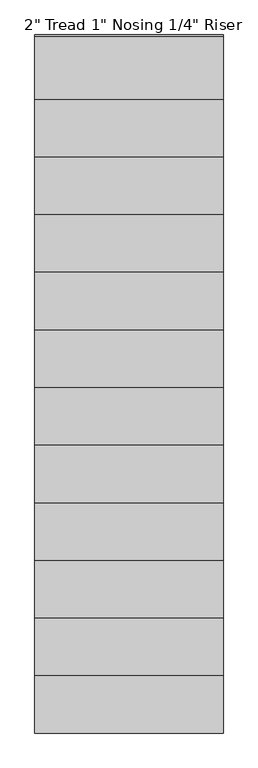
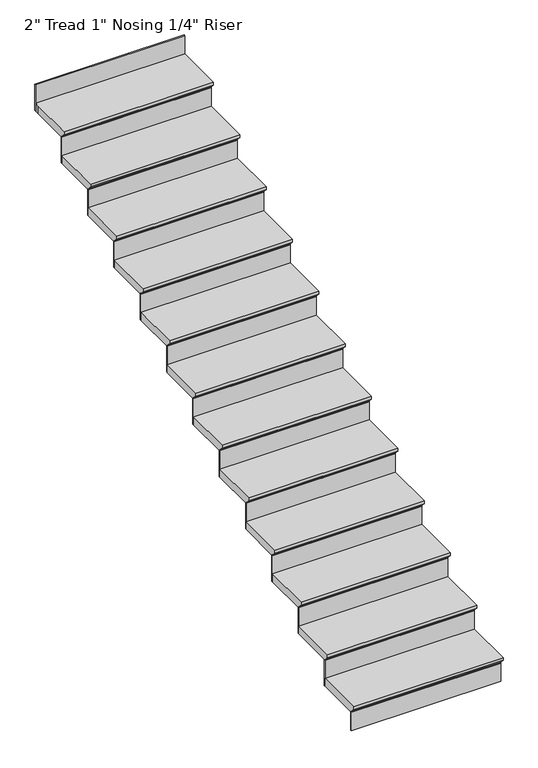
"""IFC4 building model written with IfcOpenShell, lengths in millimetres: stair flight geometry."""

from ifc_helpers import new_model, si_unit, origin, place, context, project, spatial, faceted_brep, source, transform, mapped, element, save


def stair_flight_c0f4d4ee(model_context):
    return source(origin(), model_context, "Body", "Brep", [
        faceted_brep([(-2703.0415084, 19841.9216096, 25384.9005799), (-2703.0415084, 19841.9216096, 25403.9505799), (-3617.4415084, 19841.9216096, 25403.9505799), (-3617.4415084, 19841.9216096, 25384.9005799), (-2703.0415084, 19867.3216096, 25359.5005799), (-3617.4415084, 19867.3216096, 25359.5005799), (-2703.0415084, 20146.7216096, 25403.9505799), (-3617.4415084, 20146.7216096, 25403.9505799), (-3617.4415084, 19867.3216096, 25353.1505799), (-3617.4415084, 20146.7216096, 25353.1505799), (-2703.0415084, 20146.7216096, 25353.1505799), (-2703.0415084, 19867.3216096, 25353.1505799)], [[[0, 1, 2, 3]], [[4, 0, 3, 5]], [[2, 1, 6, 7]], [[8, 9, 10, 11]], [[2, 7, 9, 8, 5, 3]], [[8, 11, 4, 5]], [[6, 1, 0, 4, 11, 10]], [[7, 6, 10, 9]]]),
        faceted_brep([(-2703.0415084, 19867.3216096, 25353.1505799), (-2703.0415084, 19867.3216096, 25234.6172466), (-2703.0415084, 19873.6716096, 25234.6172466), (-2703.0415084, 19873.6716096, 25353.1505799), (-3617.4415084, 19867.3216096, 25353.1505799), (-3617.4415084, 19873.6716096, 25353.1505799), (-3617.4415084, 19873.6716096, 25234.6172466), (-3617.4415084, 19867.3216096, 25234.6172466)], [[[0, 1, 2, 3]], [[4, 5, 6, 7]], [[1, 0, 4, 7]], [[2, 1, 7, 6]], [[3, 2, 6, 5]], [[0, 3, 5, 4]]]),
        faceted_brep([(-2703.0415084, 20146.7216096, 25522.4839133), (-2703.0415084, 20146.7216096, 25353.1505799), (-2703.0415084, 20153.0716096, 25353.1505799), (-2703.0415084, 20153.0716096, 25522.4839133), (-3617.4415084, 20146.7216096, 25522.4839133), (-3617.4415084, 20153.0716096, 25522.4839133), (-3617.4415084, 20153.0716096, 25353.1505799), (-3617.4415084, 20146.7216096, 25353.1505799)], [[[0, 1, 2, 3]], [[4, 5, 6, 7]], [[1, 0, 4, 7]], [[2, 1, 7, 6]], [[3, 2, 6, 5]], [[0, 3, 5, 4]]]),
        faceted_brep([(-3617.4415084, 20121.3216096, 25573.2839133), (-2703.0415084, 20121.3216096, 25573.2839133), (-2703.0415084, 20426.1216096, 25573.2839133), (-3617.4415084, 20426.1216096, 25573.2839133), (-3617.4415084, 20146.7216096, 25522.4839133), (-3617.4415084, 20426.1216096, 25522.4839133), (-2703.0415084, 20426.1216096, 25522.4839133), (-2703.0415084, 20146.7216096, 25522.4839133), (-3617.4415084, 20146.7216096, 25528.8339133), (-3617.4415084, 20121.3216096, 25554.2339133), (-2703.0415084, 20146.7216096, 25528.8339133), (-2703.0415084, 20121.3216096, 25554.2339133)], [[[0, 1, 2, 3]], [[4, 5, 6, 7]], [[0, 3, 5, 4, 8, 9]], [[4, 7, 10, 8]], [[2, 1, 11, 10, 7, 6]], [[3, 2, 6, 5]], [[11, 1, 0, 9]], [[10, 11, 9, 8]]]),
        faceted_brep([(-2703.0415084, 20426.1216096, 25691.8172466), (-2703.0415084, 20426.1216096, 25522.4839133), (-2703.0415084, 20432.4716096, 25522.4839133), (-2703.0415084, 20432.4716096, 25691.8172466), (-3617.4415084, 20426.1216096, 25691.8172466), (-3617.4415084, 20432.4716096, 25691.8172466), (-3617.4415084, 20432.4716096, 25522.4839133), (-3617.4415084, 20426.1216096, 25522.4839133)], [[[0, 1, 2, 3]], [[4, 5, 6, 7]], [[1, 0, 4, 7]], [[2, 1, 7, 6]], [[3, 2, 6, 5]], [[0, 3, 5, 4]]]),
        faceted_brep([(-3617.4415084, 20400.7216096, 25742.6172466), (-2703.0415084, 20400.7216096, 25742.6172466), (-2703.0415084, 20705.5216096, 25742.6172466), (-3617.4415084, 20705.5216096, 25742.6172466), (-3617.4415084, 20426.1216096, 25691.8172466), (-3617.4415084, 20705.5216096, 25691.8172466), (-2703.0415084, 20705.5216096, 25691.8172466), (-2703.0415084, 20426.1216096, 25691.8172466), (-3617.4415084, 20426.1216096, 25698.1672466), (-3617.4415084, 20400.7216096, 25723.5672466), (-2703.0415084, 20426.1216096, 25698.1672466), (-2703.0415084, 20400.7216096, 25723.5672466)], [[[0, 1, 2, 3]], [[4, 5, 6, 7]], [[0, 3, 5, 4, 8, 9]], [[4, 7, 10, 8]], [[2, 1, 11, 10, 7, 6]], [[3, 2, 6, 5]], [[11, 1, 0, 9]], [[10, 11, 9, 8]]]),
        faceted_brep([(-2703.0415084, 20705.5216096, 25861.1505799), (-2703.0415084, 20705.5216096, 25691.8172466), (-2703.0415084, 20711.8716096, 25691.8172466), (-2703.0415084, 20711.8716096, 25861.1505799), (-3617.4415084, 20705.5216096, 25861.1505799), (-3617.4415084, 20711.8716096, 25861.1505799), (-3617.4415084, 20711.8716096, 25691.8172466), (-3617.4415084, 20705.5216096, 25691.8172466)], [[[0, 1, 2, 3]], [[4, 5, 6, 7]], [[1, 0, 4, 7]], [[2, 1, 7, 6]], [[3, 2, 6, 5]], [[0, 3, 5, 4]]]),
        faceted_brep([(-3617.4415084, 20680.1216096, 25911.9505799), (-2703.0415084, 20680.1216096, 25911.9505799), (-2703.0415084, 20984.9216096, 25911.9505799), (-3617.4415084, 20984.9216096, 25911.9505799), (-3617.4415084, 20705.5216096, 25861.1505799), (-3617.4415084, 20984.9216096, 25861.1505799), (-2703.0415084, 20984.9216096, 25861.1505799), (-2703.0415084, 20705.5216096, 25861.1505799), (-3617.4415084, 20705.5216096, 25867.5005799), (-3617.4415084, 20680.1216096, 25892.9005799), (-2703.0415084, 20705.5216096, 25867.5005799), (-2703.0415084, 20680.1216096, 25892.9005799)], [[[0, 1, 2, 3]], [[4, 5, 6, 7]], [[0, 3, 5, 4, 8, 9]], [[4, 7, 10, 8]], [[2, 1, 11, 10, 7, 6]], [[3, 2, 6, 5]], [[11, 1, 0, 9]], [[10, 11, 9, 8]]]),
        faceted_brep([(-2703.0415084, 20984.9216096, 26030.4839133), (-2703.0415084, 20984.9216096, 25861.1505799), (-2703.0415084, 20991.2716096, 25861.1505799), (-2703.0415084, 20991.2716096, 26030.4839133), (-3617.4415084, 20984.9216096, 26030.4839133), (-3617.4415084, 20991.2716096, 26030.4839133), (-3617.4415084, 20991.2716096, 25861.1505799), (-3617.4415084, 20984.9216096, 25861.1505799)], [[[0, 1, 2, 3]], [[4, 5, 6, 7]], [[1, 0, 4, 7]], [[2, 1, 7, 6]], [[3, 2, 6, 5]], [[0, 3, 5, 4]]]),
        faceted_brep([(-3617.4415084, 20959.5216096, 26081.2839133), (-2703.0415084, 20959.5216096, 26081.2839133), (-2703.0415084, 21264.3216096, 26081.2839133), (-3617.4415084, 21264.3216096, 26081.2839133), (-3617.4415084, 20984.9216096, 26030.4839133), (-3617.4415084, 21264.3216096, 26030.4839133), (-2703.0415084, 21264.3216096, 26030.4839133), (-2703.0415084, 20984.9216096, 26030.4839133), (-3617.4415084, 20984.9216096, 26036.8339133), (-3617.4415084, 20959.5216096, 26062.2339133), (-2703.0415084, 20984.9216096, 26036.8339133), (-2703.0415084, 20959.5216096, 26062.2339133)], [[[0, 1, 2, 3]], [[4, 5, 6, 7]], [[0, 3, 5, 4, 8, 9]], [[4, 7, 10, 8]], [[2, 1, 11, 10, 7, 6]], [[3, 2, 6, 5]], [[11, 1, 0, 9]], [[10, 11, 9, 8]]]),
        faceted_brep([(-2703.0415084, 21264.3216096, 26199.8172466), (-2703.0415084, 21264.3216096, 26030.4839133), (-2703.0415084, 21270.6716096, 26030.4839133), (-2703.0415084, 21270.6716096, 26199.8172466), (-3617.4415084, 21264.3216096, 26199.8172466), (-3617.4415084, 21270.6716096, 26199.8172466), (-3617.4415084, 21270.6716096, 26030.4839133), (-3617.4415084, 21264.3216096, 26030.4839133)], [[[0, 1, 2, 3]], [[4, 5, 6, 7]], [[1, 0, 4, 7]], [[2, 1, 7, 6]], [[3, 2, 6, 5]], [[0, 3, 5, 4]]]),
        faceted_brep([(-3617.4415084, 21238.9216096, 26250.6172466), (-2703.0415084, 21238.9216096, 26250.6172466), (-2703.0415084, 21543.7216096, 26250.6172466), (-3617.4415084, 21543.7216096, 26250.6172466), (-3617.4415084, 21264.3216096, 26199.8172466), (-3617.4415084, 21543.7216096, 26199.8172466), (-2703.0415084, 21543.7216096, 26199.8172466), (-2703.0415084, 21264.3216096, 26199.8172466), (-3617.4415084, 21264.3216096, 26206.1672466), (-3617.4415084, 21238.9216096, 26231.5672466), (-2703.0415084, 21264.3216096, 26206.1672466), (-2703.0415084, 21238.9216096, 26231.5672466)], [[[0, 1, 2, 3]], [[4, 5, 6, 7]], [[0, 3, 5, 4, 8, 9]], [[4, 7, 10, 8]], [[2, 1, 11, 10, 7, 6]], [[3, 2, 6, 5]], [[11, 1, 0, 9]], [[10, 11, 9, 8]]]),
        faceted_brep([(-2703.0415084, 21543.7216096, 26369.1505799), (-2703.0415084, 21543.7216096, 26199.8172466), (-2703.0415084, 21550.0716096, 26199.8172466), (-2703.0415084, 21550.0716096, 26369.1505799), (-3617.4415084, 21543.7216096, 26369.1505799), (-3617.4415084, 21550.0716096, 26369.1505799), (-3617.4415084, 21550.0716096, 26199.8172466), (-3617.4415084, 21543.7216096, 26199.8172466)], [[[0, 1, 2, 3]], [[4, 5, 6, 7]], [[1, 0, 4, 7]], [[2, 1, 7, 6]], [[3, 2, 6, 5]], [[0, 3, 5, 4]]]),
        faceted_brep([(-3617.4415084, 21518.3216096, 26419.9505799), (-2703.0415084, 21518.3216096, 26419.9505799), (-2703.0415084, 21823.1216096, 26419.9505799), (-3617.4415084, 21823.1216096, 26419.9505799), (-3617.4415084, 21543.7216096, 26369.1505799), (-3617.4415084, 21823.1216096, 26369.1505799), (-2703.0415084, 21823.1216096, 26369.1505799), (-2703.0415084, 21543.7216096, 26369.1505799), (-3617.4415084, 21543.7216096, 26375.5005799), (-3617.4415084, 21518.3216096, 26400.9005799), (-2703.0415084, 21543.7216096, 26375.5005799), (-2703.0415084, 21518.3216096, 26400.9005799)], [[[0, 1, 2, 3]], [[4, 5, 6, 7]], [[0, 3, 5, 4, 8, 9]], [[4, 7, 10, 8]], [[2, 1, 11, 10, 7, 6]], [[3, 2, 6, 5]], [[11, 1, 0, 9]], [[10, 11, 9, 8]]]),
        faceted_brep([(-2703.0415084, 21823.1216096, 26538.4839133), (-2703.0415084, 21823.1216096, 26369.1505799), (-2703.0415084, 21829.4716096, 26369.1505799), (-2703.0415084, 21829.4716096, 26538.4839133), (-3617.4415084, 21823.1216096, 26538.4839133), (-3617.4415084, 21829.4716096, 26538.4839133), (-3617.4415084, 21829.4716096, 26369.1505799), (-3617.4415084, 21823.1216096, 26369.1505799)], [[[0, 1, 2, 3]], [[4, 5, 6, 7]], [[1, 0, 4, 7]], [[2, 1, 7, 6]], [[3, 2, 6, 5]], [[0, 3, 5, 4]]]),
        faceted_brep([(-3617.4415084, 21797.7216096, 26589.2839133), (-2703.0415084, 21797.7216096, 26589.2839133), (-2703.0415084, 22102.5216096, 26589.2839133), (-3617.4415084, 22102.5216096, 26589.2839133), (-3617.4415084, 21823.1216096, 26538.4839133), (-3617.4415084, 22102.5216096, 26538.4839133), (-2703.0415084, 22102.5216096, 26538.4839133), (-2703.0415084, 21823.1216096, 26538.4839133), (-3617.4415084, 21823.1216096, 26544.8339133), (-3617.4415084, 21797.7216096, 26570.2339133), (-2703.0415084, 21823.1216096, 26544.8339133), (-2703.0415084, 21797.7216096, 26570.2339133)], [[[0, 1, 2, 3]], [[4, 5, 6, 7]], [[0, 3, 5, 4, 8, 9]], [[4, 7, 10, 8]], [[2, 1, 11, 10, 7, 6]], [[3, 2, 6, 5]], [[11, 1, 0, 9]], [[10, 11, 9, 8]]]),
        faceted_brep([(-2703.0415084, 22102.5216096, 26707.8172466), (-2703.0415084, 22102.5216096, 26538.4839133), (-2703.0415084, 22108.8716096, 26538.4839133), (-2703.0415084, 22108.8716096, 26707.8172466), (-3617.4415084, 22102.5216096, 26707.8172466), (-3617.4415084, 22108.8716096, 26707.8172466), (-3617.4415084, 22108.8716096, 26538.4839133), (-3617.4415084, 22102.5216096, 26538.4839133)], [[[0, 1, 2, 3]], [[4, 5, 6, 7]], [[1, 0, 4, 7]], [[2, 1, 7, 6]], [[3, 2, 6, 5]], [[0, 3, 5, 4]]]),
        faceted_brep([(-3617.4415084, 22077.1216096, 26758.6172466), (-2703.0415084, 22077.1216096, 26758.6172466), (-2703.0415084, 22381.9216096, 26758.6172466), (-3617.4415084, 22381.9216096, 26758.6172466), (-3617.4415084, 22102.5216096, 26707.8172466), (-3617.4415084, 22381.9216096, 26707.8172466), (-2703.0415084, 22381.9216096, 26707.8172466), (-2703.0415084, 22102.5216096, 26707.8172466), (-3617.4415084, 22102.5216096, 26714.1672466), (-3617.4415084, 22077.1216096, 26739.5672466), (-2703.0415084, 22102.5216096, 26714.1672466), (-2703.0415084, 22077.1216096, 26739.5672466)], [[[0, 1, 2, 3]], [[4, 5, 6, 7]], [[0, 3, 5, 4, 8, 9]], [[4, 7, 10, 8]], [[2, 1, 11, 10, 7, 6]], [[3, 2, 6, 5]], [[11, 1, 0, 9]], [[10, 11, 9, 8]]]),
        faceted_brep([(-2703.0415084, 22381.9216096, 26877.1505799), (-2703.0415084, 22381.9216096, 26707.8172466), (-2703.0415084, 22388.2716096, 26707.8172466), (-2703.0415084, 22388.2716096, 26877.1505799), (-3617.4415084, 22381.9216096, 26877.1505799), (-3617.4415084, 22388.2716096, 26877.1505799), (-3617.4415084, 22388.2716096, 26707.8172466), (-3617.4415084, 22381.9216096, 26707.8172466)], [[[0, 1, 2, 3]], [[4, 5, 6, 7]], [[1, 0, 4, 7]], [[2, 1, 7, 6]], [[3, 2, 6, 5]], [[0, 3, 5, 4]]]),
        faceted_brep([(-3617.4415084, 22356.5216096, 26927.9505799), (-2703.0415084, 22356.5216096, 26927.9505799), (-2703.0415084, 22661.3216096, 26927.9505799), (-3617.4415084, 22661.3216096, 26927.9505799), (-3617.4415084, 22381.9216096, 26877.1505799), (-3617.4415084, 22661.3216096, 26877.1505799), (-2703.0415084, 22661.3216096, 26877.1505799), (-2703.0415084, 22381.9216096, 26877.1505799), (-3617.4415084, 22381.9216096, 26883.5005799), (-3617.4415084, 22356.5216096, 26908.9005799), (-2703.0415084, 22381.9216096, 26883.5005799), (-2703.0415084, 22356.5216096, 26908.9005799)], [[[0, 1, 2, 3]], [[4, 5, 6, 7]], [[0, 3, 5, 4, 8, 9]], [[4, 7, 10, 8]], [[2, 1, 11, 10, 7, 6]], [[3, 2, 6, 5]], [[11, 1, 0, 9]], [[10, 11, 9, 8]]]),
        faceted_brep([(-2703.0415084, 22661.3216096, 27046.4839133), (-2703.0415084, 22661.3216096, 26877.1505799), (-2703.0415084, 22667.6716096, 26877.1505799), (-2703.0415084, 22667.6716096, 27046.4839133), (-3617.4415084, 22661.3216096, 27046.4839133), (-3617.4415084, 22667.6716096, 27046.4839133), (-3617.4415084, 22667.6716096, 26877.1505799), (-3617.4415084, 22661.3216096, 26877.1505799)], [[[0, 1, 2, 3]], [[4, 5, 6, 7]], [[1, 0, 4, 7]], [[2, 1, 7, 6]], [[3, 2, 6, 5]], [[0, 3, 5, 4]]]),
        faceted_brep([(-3617.4415084, 22635.9216096, 27097.2839133), (-2703.0415084, 22635.9216096, 27097.2839133), (-2703.0415084, 22940.7216096, 27097.2839133), (-3617.4415084, 22940.7216096, 27097.2839133), (-3617.4415084, 22661.3216096, 27046.4839133), (-3617.4415084, 22940.7216096, 27046.4839133), (-2703.0415084, 22940.7216096, 27046.4839133), (-2703.0415084, 22661.3216096, 27046.4839133), (-3617.4415084, 22661.3216096, 27052.8339133), (-3617.4415084, 22635.9216096, 27078.2339133), (-2703.0415084, 22661.3216096, 27052.8339133), (-2703.0415084, 22635.9216096, 27078.2339133)], [[[0, 1, 2, 3]], [[4, 5, 6, 7]], [[0, 3, 5, 4, 8, 9]], [[4, 7, 10, 8]], [[2, 1, 11, 10, 7, 6]], [[3, 2, 6, 5]], [[11, 1, 0, 9]], [[10, 11, 9, 8]]]),
        faceted_brep([(-2703.0415084, 23220.1216096, 27385.1505799), (-2703.0415084, 23220.1216096, 27215.8172466), (-2703.0415084, 23226.4716096, 27215.8172466), (-2703.0415084, 23226.4716096, 27385.1505799), (-3617.4415084, 23220.1216096, 27385.1505799), (-3617.4415084, 23226.4716096, 27385.1505799), (-3617.4415084, 23226.4716096, 27215.8172466), (-3617.4415084, 23220.1216096, 27215.8172466)], [[[0, 1, 2, 3]], [[4, 5, 6, 7]], [[1, 0, 4, 7]], [[2, 1, 7, 6]], [[3, 2, 6, 5]], [[0, 3, 5, 4]]]),
        faceted_brep([(-2703.0415084, 22940.7216096, 27215.8172466), (-2703.0415084, 22940.7216096, 27046.4839133), (-2703.0415084, 22947.0716096, 27046.4839133), (-2703.0415084, 22947.0716096, 27215.8172466), (-3617.4415084, 22940.7216096, 27215.8172466), (-3617.4415084, 22947.0716096, 27215.8172466), (-3617.4415084, 22947.0716096, 27046.4839133), (-3617.4415084, 22940.7216096, 27046.4839133)], [[[0, 1, 2, 3]], [[4, 5, 6, 7]], [[1, 0, 4, 7]], [[2, 1, 7, 6]], [[3, 2, 6, 5]], [[0, 3, 5, 4]]]),
        faceted_brep([(-3617.4415084, 23220.1216096, 27266.6172466), (-3617.4415084, 23194.7216096, 27266.6172466), (-3617.4415084, 22915.3216096, 27266.6172466), (-2703.0415084, 22915.3216096, 27266.6172466), (-2703.0415084, 23220.1216096, 27266.6172466), (-3617.4415084, 23194.7216096, 27215.8172466), (-3617.4415084, 23220.1216096, 27215.8172466), (-2703.0415084, 23220.1216096, 27215.8172466), (-2703.0415084, 22940.7216096, 27215.8172466), (-3617.4415084, 22940.7216096, 27215.8172466), (-3617.4415084, 22940.7216096, 27222.1672466), (-3617.4415084, 22915.3216096, 27247.5672466), (-2703.0415084, 22940.7216096, 27222.1672466), (-2703.0415084, 22915.3216096, 27247.5672466)], [[[0, 1, 2, 3, 4]], [[5, 6, 7, 8, 9]], [[1, 0, 6, 5]], [[2, 1, 5, 9, 10, 11]], [[9, 8, 12, 10]], [[4, 3, 13, 12, 8, 7]], [[0, 4, 7, 6]], [[13, 3, 2, 11]], [[12, 13, 11, 10]]]),
    ])


if __name__ == "__main__":
    model = new_model("IFC4")
    model_context = context("Model", 3, world=origin())
    ifc_project = project(units=[si_unit("LENGTHUNIT", "METRE", prefix="MILLI")], contexts=[model_context])
    site = spatial("IfcSite", under=ifc_project)
    building = spatial("IfcBuilding", under=site)
    placement = place(None, origin())
    stair_flight_shape = stair_flight_c0f4d4ee(model_context)
    element("IfcStairFlight", 1, ObjectType="2\" Tread 1\" Nosing 1/4\" Riser", at=placement, inside=building, context=model_context, shape_type="MappedRepresentation", body=[
        mapped(stair_flight_shape, transform((0.0, 0.0, 0.0), x_axis=(1.0, 0.0, 0.0), y_axis=(0.0, 1.0, 0.0), z_axis=(0.0, 0.0, 1.0))),
    ])
    save(model, "model.ifc")
